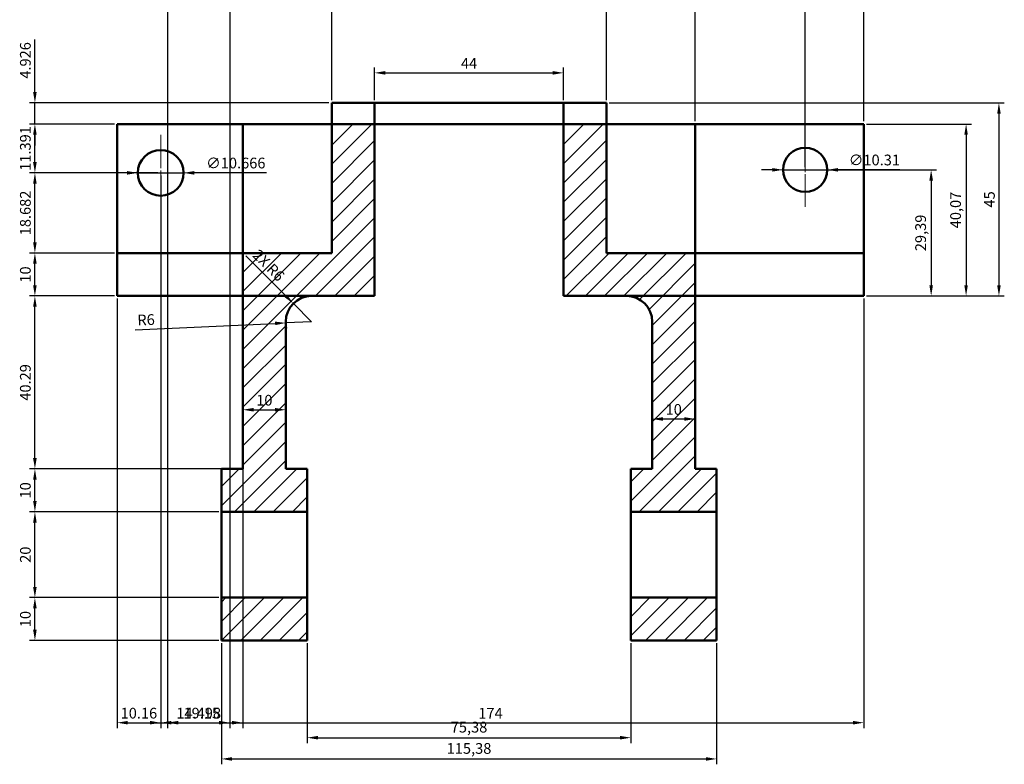
# Model space of a CAD drawing. Units: millimetres. Extents: x 2172 to 2566, y 897 to 1244.
# Tile 1 of 3: x 2172 to 2402, y 897 to 1071. Entities that reach past the tile are written whole.
import ezdxf

# ---------------------------------------------------------------- set-up
doc = ezdxf.new("R2010")
doc.units = ezdxf.units.MM
doc.linetypes.add('CENTER', pattern=[50.8, 31.75, -6.35, 6.35, -6.35])
for name, color, linetype, lineweight in [('M-CNTR', 4, 'CENTER', 18), ('M-DIMS', 2, 'Continuous', 25), ('M-HATC', 8, 'Continuous', 18), ('M-OUTL', 7, 'Continuous', 50)]:
    doc.layers.add(name, color=color, linetype=linetype, lineweight=lineweight)
doc.styles.get("Standard").update_dxf_attribs({"font": 'arial.ttf'})
doc.dimstyles.new('ISO-25', dxfattribs={"dimtxt": 2.5, "dimasz": 2.5, "dimexe": 1.25, "dimexo": 0.625, "dimtad": 1, "dimtxsty": 'Standard', "dimcen": 2.5, "dimadec": 0, "dimazin": 0, "dimtfac": 1, "dimtmove": 0, "dimatfit": 3, "dimfxl": 1, "dimarcsym": 0})

# ---------------------------------------------------------------- blocks, each defined once
blk = doc.blocks.new('*U1')
at = {"layer": 'M-CNTR', "color": 0, "transparency": 16777216}
for p, q in [((0, 1.07), (0, 8.83)), ((-8.83, 0), (-1.07, 0)), ((1.07, 0), (8.83, 0)), ((0, -8.83), (0, -1.07))]:
    blk.add_line(p, q, dxfattribs=at)
at = {"layer": 'M-CNTR', "color": 0, "linetype": 'Continuous', "transparency": 16777216}
for p, q in [((-0.53, 0), (0.53, 0)), ((0, -0.53), (0, 0.53))]:
    blk.add_line(p, q, dxfattribs=at)
blk = doc.blocks.new('*U2')
at = {"layer": 'M-CNTR', "color": 0, "transparency": 16777216}
for p, q in [((0, 1.03), (0, 8.66)), ((-8.66, 0), (-1.03, 0)), ((1.03, 0), (8.66, 0)), ((0, -8.66), (0, -1.03))]:
    blk.add_line(p, q, dxfattribs=at)
at = {"layer": 'M-CNTR', "color": 0, "linetype": 'Continuous', "transparency": 16777216}
for p, q in [((-0.52, 0), (0.52, 0)), ((0, -0.52), (0, 0.52))]:
    blk.add_line(p, q, dxfattribs=at)
blk = doc.blocks.new('*D10')
at = {"layer": 'Defpoints', "color": 0, "transparency": 16777216}
for p in [(2219.1, 925.96), (2334.48, 925.96), (2334.48, 898.37)]:
    blk.add_point(p, dxfattribs=at)
at = {"layer": 'M-DIMS', "color": 0, "lineweight": -2, "transparency": 16777216}
for p, q in [((2219.1, 925.34), (2219.1, 897.12)), ((2334.48, 925.34), (2334.48, 897.12)), ((2221.6, 898.37), (2331.98, 898.37))]:
    blk.add_line(p, q, dxfattribs=at)
at = {"layer": 'M-DIMS', "color": 0, "transparency": 16777216}
for points in [[(2221.6, 898.78), (2221.6, 897.95), (2219.1, 898.37)], [(2331.98, 898.78), (2331.98, 897.95), (2334.48, 898.37)]]:
    blk.add_solid(points, dxfattribs=at)
at = {"layer": 'M-DIMS', "color": 0, "transparency": 16777216, "insert": (2276.79, 900.49), "char_height": 2.5, "attachment_point": 5}
blk.add_mtext('115,38', dxfattribs=at)
blk = doc.blocks.new('*D11')
at = {"layer": 'Defpoints', "color": 0, "transparency": 16777216}
for p in [(2239.1, 925.96), (2314.48, 925.96), (2314.48, 903.32)]:
    blk.add_point(p, dxfattribs=at)
at = {"layer": 'M-DIMS', "color": 0, "lineweight": -2, "transparency": 16777216}
for p, q in [((2239.1, 925.34), (2239.1, 902.07)), ((2314.48, 925.34), (2314.48, 902.07)), ((2241.6, 903.32), (2311.98, 903.32))]:
    blk.add_line(p, q, dxfattribs=at)
at = {"layer": 'M-DIMS', "color": 0, "transparency": 16777216}
for points in [[(2241.6, 903.74), (2241.6, 902.9), (2239.1, 903.32)], [(2311.98, 903.74), (2311.98, 902.9), (2314.48, 903.32)]]:
    blk.add_solid(points, dxfattribs=at)
at = {"layer": 'M-DIMS', "color": 0, "transparency": 16777216, "insert": (2276.79, 905.45), "char_height": 2.5, "attachment_point": 5}
blk.add_mtext('75,38', dxfattribs=at)
blk = doc.blocks.new('*D12')
at = {"layer": 'Defpoints', "color": 0, "transparency": 16777216}
for p in [(2224.1, 986.11), (2234.1, 983.11), (2234.1, 979.74)]:
    blk.add_point(p, dxfattribs=at)
at = {"layer": 'M-DIMS', "color": 0, "lineweight": -2, "transparency": 16777216}
for p, q in [((2224.1, 985.48), (2224.1, 978.49)), ((2234.1, 982.48), (2234.1, 978.49)), ((2226.6, 979.74), (2231.6, 979.74))]:
    blk.add_line(p, q, dxfattribs=at)
at = {"layer": 'M-DIMS', "color": 0, "transparency": 16777216}
for points in [[(2226.6, 980.16), (2226.6, 979.32), (2224.1, 979.74)], [(2231.6, 980.16), (2231.6, 979.32), (2234.1, 979.74)]]:
    blk.add_solid(points, dxfattribs=at)
at = {"layer": 'M-DIMS', "color": 0, "transparency": 16777216, "insert": (2229.1, 981.64), "char_height": 2.5, "attachment_point": 5}
blk.add_mtext('10', dxfattribs=at)
blk = doc.blocks.new('*D13')
at = {"layer": 'Defpoints', "color": 0, "transparency": 16777216}
for p in [(2329.48, 986.11), (2319.48, 983.11), (2329.48, 977.59)]:
    blk.add_point(p, dxfattribs=at)
at = {"layer": 'M-DIMS', "color": 0, "lineweight": -2, "transparency": 16777216}
for p, q in [((2329.48, 985.48), (2329.48, 976.34)), ((2319.48, 982.48), (2319.48, 976.34)), ((2321.98, 977.59), (2326.98, 977.59))]:
    blk.add_line(p, q, dxfattribs=at)
at = {"layer": 'M-DIMS', "color": 0, "transparency": 16777216}
for points in [[(2321.98, 978.01), (2321.98, 977.17), (2319.48, 977.59)], [(2326.98, 978.01), (2326.98, 977.17), (2329.48, 977.59)]]:
    blk.add_solid(points, dxfattribs=at)
at = {"layer": 'M-DIMS', "color": 0, "transparency": 16777216, "insert": (2324.48, 979.49), "char_height": 2.5, "attachment_point": 5}
blk.add_mtext('10', dxfattribs=at)
blk = doc.blocks.new('*D14')
at = {"layer": 'Defpoints', "color": 0, "transparency": 16777216}
for p in [(2355.12, 1035.65), (2368.79, 1006.26), (2384.47, 1006.26)]:
    blk.add_point(p, dxfattribs=at)
at = {"layer": 'M-DIMS', "color": 0, "lineweight": -2, "transparency": 16777216}
for p, q in [((2355.75, 1035.65), (2385.72, 1035.65)), ((2384.47, 1033.15), (2384.47, 1008.76)), ((2369.41, 1006.26), (2385.72, 1006.26))]:
    blk.add_line(p, q, dxfattribs=at)
at = {"layer": 'M-DIMS', "color": 0, "transparency": 16777216}
for points in [[(2384.05, 1033.15), (2384.89, 1033.15), (2384.47, 1035.65)], [(2384.05, 1008.76), (2384.89, 1008.76), (2384.47, 1006.26)]]:
    blk.add_solid(points, dxfattribs=at)
at = {"layer": 'M-DIMS', "color": 0, "transparency": 16777216, "insert": (2382.34, 1020.95), "char_height": 2.5, "attachment_point": 5, "rotation": 90}
blk.add_mtext('29,39', dxfattribs=at)
blk = doc.blocks.new('*D15')
at = {"layer": 'Defpoints', "color": 0, "transparency": 16777216}
for p in [(2368.79, 1046.33), (2368.79, 1006.26), (2392.61, 1006.26)]:
    blk.add_point(p, dxfattribs=at)
at = {"layer": 'M-DIMS', "color": 0, "lineweight": -2, "transparency": 16777216}
for p, q in [((2369.41, 1046.33), (2393.86, 1046.33)), ((2392.61, 1043.83), (2392.61, 1008.76)), ((2369.41, 1006.26), (2393.86, 1006.26))]:
    blk.add_line(p, q, dxfattribs=at)
at = {"layer": 'M-DIMS', "color": 0, "transparency": 16777216}
for points in [[(2392.19, 1043.83), (2393.02, 1043.83), (2392.61, 1046.33)], [(2392.19, 1008.76), (2393.02, 1008.76), (2392.61, 1006.26)]]:
    blk.add_solid(points, dxfattribs=at)
at = {"layer": 'M-DIMS', "color": 0, "transparency": 16777216, "insert": (2390.48, 1026.29), "char_height": 2.5, "attachment_point": 5, "rotation": 90}
blk.add_mtext('40,07', dxfattribs=at)
blk = doc.blocks.new('*D16')
at = {"layer": 'Defpoints', "color": 0, "transparency": 16777216}
for p in [(2308.79, 1051.26), (2368.79, 1006.26), (2400.26, 1006.26)]:
    blk.add_point(p, dxfattribs=at)
at = {"layer": 'M-DIMS', "color": 0, "lineweight": -2, "transparency": 16777216}
for p, q in [((2309.41, 1051.26), (2401.51, 1051.26)), ((2400.26, 1048.76), (2400.26, 1008.76)), ((2369.41, 1006.26), (2401.51, 1006.26))]:
    blk.add_line(p, q, dxfattribs=at)
at = {"layer": 'M-DIMS', "color": 0, "transparency": 16777216}
for points in [[(2399.85, 1048.76), (2400.68, 1048.76), (2400.26, 1051.26)], [(2399.85, 1008.76), (2400.68, 1008.76), (2400.26, 1006.26)]]:
    blk.add_solid(points, dxfattribs=at)
at = {"layer": 'M-DIMS', "color": 0, "transparency": 16777216, "insert": (2398.37, 1028.76), "char_height": 2.5, "attachment_point": 5, "rotation": 90}
blk.add_mtext('45', dxfattribs=at)
blk = doc.blocks.new('*D17')
at = {"layer": 'Defpoints', "color": 0, "transparency": 16777216}
for p in [(2298.79, 1058.25), (2254.79, 1051.26), (2298.79, 1051.26)]:
    blk.add_point(p, dxfattribs=at)
at = {"layer": 'M-DIMS', "color": 0, "lineweight": -2, "transparency": 16777216}
for p, q in [((2254.79, 1051.88), (2254.79, 1059.5)), ((2257.29, 1058.25), (2296.29, 1058.25)), ((2298.79, 1051.88), (2298.79, 1059.5))]:
    blk.add_line(p, q, dxfattribs=at)
at = {"layer": 'M-DIMS', "color": 0, "transparency": 16777216}
for points in [[(2257.29, 1058.67), (2257.29, 1057.83), (2254.79, 1058.25)], [(2296.29, 1058.67), (2296.29, 1057.83), (2298.79, 1058.25)]]:
    blk.add_solid(points, dxfattribs=at)
at = {"layer": 'M-DIMS', "color": 0, "transparency": 16777216, "insert": (2276.79, 1060.13), "char_height": 2.5, "attachment_point": 5}
blk.add_mtext('44', dxfattribs=at)
blk = doc.blocks.new('*D18')
at = {"layer": 'Defpoints', "color": 0, "transparency": 16777216}
for p in [(2234.1, 999.98), (2240.1, 1000.26)]:
    blk.add_point(p, dxfattribs=at)
at = {"layer": 'M-DIMS', "color": 0, "lineweight": -2, "transparency": 16777216}
for p, q in [((2199, 998.36), (2231.61, 999.86)), ((2240.1, 1000.26), (2234.1, 999.98))]:
    blk.add_line(p, q, dxfattribs=at)
blk.add_arc((2240.1, 1000.26), 6, 180, 194.5824, dxfattribs=at)
at = {"layer": 'M-DIMS', "color": 0, "transparency": 16777216}
blk.add_solid([(2231.59, 1000.28), (2231.63, 999.45), (2234.1, 999.98)], dxfattribs=at)
at = {"layer": 'M-DIMS', "color": 0, "transparency": 16777216, "insert": (2201.55, 1000.38), "char_height": 2.5, "attachment_point": 5, "rotation": 2.6458}
blk.add_mtext('R6', dxfattribs=at)
blk = doc.blocks.new('*D40')
at = {"layer": 'Defpoints', "color": 0, "transparency": 16777216}
for p in [(2206.56, 1172.22), (2221.06, 1154.78), (2221.06, 906.81)]:
    blk.add_point(p, dxfattribs=at)
at = {"layer": 'M-DIMS', "color": 0, "lineweight": -2, "transparency": 16777216}
for p, q in [((2206.56, 1171.6), (2206.56, 905.56)), ((2221.06, 1154.15), (2221.06, 905.56)), ((2209.06, 906.81), (2218.56, 906.81))]:
    blk.add_line(p, q, dxfattribs=at)
at = {"layer": 'M-DIMS', "color": 0, "transparency": 16777216}
for points in [[(2209.06, 907.23), (2209.06, 906.4), (2206.56, 906.81)], [(2218.56, 907.23), (2218.56, 906.4), (2221.06, 906.81)]]:
    blk.add_solid(points, dxfattribs=at)
at = {"layer": 'M-DIMS', "color": 0, "transparency": 16777216, "insert": (2213.81, 908.71), "char_height": 2.5, "attachment_point": 5}
blk.add_mtext('14.498', dxfattribs=at)
blk = doc.blocks.new('*D41')
at = {"layer": 'Defpoints', "color": 0, "transparency": 16777216}
for p in [(2194.79, 1006.26), (2368.79, 1006.26), (2368.79, 906.81)]:
    blk.add_point(p, dxfattribs=at)
at = {"layer": 'M-DIMS', "color": 0, "lineweight": -2, "transparency": 16777216}
for p, q in [((2194.79, 1005.63), (2194.79, 905.56)), ((2368.79, 1005.63), (2368.79, 905.56)), ((2197.29, 906.81), (2366.29, 906.81))]:
    blk.add_line(p, q, dxfattribs=at)
at = {"layer": 'M-DIMS', "color": 0, "transparency": 16777216}
for points in [[(2197.29, 907.23), (2197.29, 906.4), (2194.79, 906.81)], [(2366.29, 907.23), (2366.29, 906.4), (2368.79, 906.81)]]:
    blk.add_solid(points, dxfattribs=at)
at = {"layer": 'M-DIMS', "color": 0, "transparency": 16777216, "insert": (2281.79, 908.69), "char_height": 2.5, "attachment_point": 5}
blk.add_mtext('174', dxfattribs=at)
blk = doc.blocks.new('*D42')
at = {"layer": 'Defpoints', "color": 0, "transparency": 16777216}
for p in [(2204.95, 1034.94), (2194.79, 1006.26), (2204.95, 906.81)]:
    blk.add_point(p, dxfattribs=at)
at = {"layer": 'M-DIMS', "color": 0, "lineweight": -2, "transparency": 16777216}
for p, q in [((2204.95, 1034.31), (2204.95, 905.56)), ((2194.79, 1005.63), (2194.79, 905.56)), ((2197.29, 906.81), (2202.45, 906.81))]:
    blk.add_line(p, q, dxfattribs=at)
at = {"layer": 'M-DIMS', "color": 0, "transparency": 16777216}
for points in [[(2197.29, 907.23), (2197.29, 906.4), (2194.79, 906.81)], [(2202.45, 907.23), (2202.45, 906.4), (2204.95, 906.81)]]:
    blk.add_solid(points, dxfattribs=at)
at = {"layer": 'M-DIMS', "color": 0, "transparency": 16777216, "insert": (2199.87, 908.71), "char_height": 2.5, "attachment_point": 5}
blk.add_mtext('10.16', dxfattribs=at)
blk = doc.blocks.new('*D43')
at = {"layer": 'Defpoints', "color": 0, "transparency": 16777216}
for p in [(2204.95, 1034.94), (2224.1, 1006.26), (2224.1, 906.81)]:
    blk.add_point(p, dxfattribs=at)
at = {"layer": 'M-DIMS', "color": 0, "lineweight": -2, "transparency": 16777216}
for p, q in [((2204.95, 1034.31), (2204.95, 905.56)), ((2224.1, 1005.63), (2224.1, 905.56)), ((2207.45, 906.81), (2221.6, 906.81))]:
    blk.add_line(p, q, dxfattribs=at)
at = {"layer": 'M-DIMS', "color": 0, "transparency": 16777216}
for points in [[(2207.45, 907.23), (2207.45, 906.4), (2204.95, 906.81)], [(2221.6, 907.23), (2221.6, 906.4), (2224.1, 906.81)]]:
    blk.add_solid(points, dxfattribs=at)
at = {"layer": 'M-DIMS', "color": 0, "transparency": 16777216, "insert": (2214.52, 908.71), "char_height": 2.5, "attachment_point": 5}
blk.add_mtext('19.15', dxfattribs=at)
blk = doc.blocks.new('*D44')
at = {"layer": 'Defpoints', "color": 0, "transparency": 16777216}
for p in [(2355.12, 1218.64), (2329.48, 1046.33), (2355.12, 1035.65)]:
    blk.add_point(p, dxfattribs=at)
at = {"layer": 'M-DIMS', "color": 0, "lineweight": -2, "transparency": 16777216}
for p, q in [((2329.48, 1046.96), (2329.48, 1219.89)), ((2331.98, 1218.64), (2352.62, 1218.64)), ((2355.12, 1036.27), (2355.12, 1219.89))]:
    blk.add_line(p, q, dxfattribs=at)
at = {"layer": 'M-DIMS', "color": 0, "transparency": 16777216}
for points in [[(2331.98, 1219.05), (2331.98, 1218.22), (2329.48, 1218.64)], [(2352.62, 1219.05), (2352.62, 1218.22), (2355.12, 1218.64)]]:
    blk.add_solid(points, dxfattribs=at)
at = {"layer": 'M-DIMS', "color": 0, "transparency": 16777216, "insert": (2342.3, 1220.54), "char_height": 2.5, "attachment_point": 5}
blk.add_mtext('25.643', dxfattribs=at)
blk = doc.blocks.new('*D45')
at = {"layer": 'Defpoints', "color": 0, "transparency": 16777216}
for p in [(2368.79, 1218.64), (2368.79, 1046.33), (2355.12, 1035.65)]:
    blk.add_point(p, dxfattribs=at)
at = {"layer": 'M-DIMS', "color": 0, "lineweight": -2, "transparency": 16777216}
for p, q in [((2355.12, 1036.27), (2355.12, 1219.89)), ((2357.62, 1218.64), (2366.29, 1218.64)), ((2368.79, 1046.96), (2368.79, 1219.89))]:
    blk.add_line(p, q, dxfattribs=at)
at = {"layer": 'M-DIMS', "color": 0, "transparency": 16777216}
for points in [[(2357.62, 1219.05), (2357.62, 1218.22), (2355.12, 1218.64)], [(2366.29, 1219.05), (2366.29, 1218.22), (2368.79, 1218.64)]]:
    blk.add_solid(points, dxfattribs=at)
at = {"layer": 'M-DIMS', "color": 0, "transparency": 16777216, "insert": (2361.95, 1220.54), "char_height": 2.5, "attachment_point": 5}
blk.add_mtext('13.668', dxfattribs=at)
blk = doc.blocks.new('*D46')
at = {"layer": 'Defpoints', "color": 0, "transparency": 16777216}
for p in [(2175.64, 935.96), (2219.1, 935.96), (2219.1, 925.96)]:
    blk.add_point(p, dxfattribs=at)
at = {"layer": 'M-DIMS', "color": 0, "lineweight": -2, "transparency": 16777216}
for p, q in [((2218.47, 935.96), (2174.39, 935.96)), ((2175.64, 928.46), (2175.64, 933.46)), ((2218.47, 925.96), (2174.39, 925.96))]:
    blk.add_line(p, q, dxfattribs=at)
at = {"layer": 'M-DIMS', "color": 0, "transparency": 16777216}
for points in [[(2175.22, 933.46), (2176.05, 933.46), (2175.64, 935.96)], [(2175.22, 928.46), (2176.05, 928.46), (2175.64, 925.96)]]:
    blk.add_solid(points, dxfattribs=at)
at = {"layer": 'M-DIMS', "color": 0, "transparency": 16777216, "insert": (2173.74, 930.96), "char_height": 2.5, "attachment_point": 5, "rotation": 90}
blk.add_mtext('10', dxfattribs=at)
blk = doc.blocks.new('*D47')
at = {"layer": 'Defpoints', "color": 0, "transparency": 16777216}
for p in [(2175.64, 955.96), (2219.1, 955.96), (2219.1, 935.96)]:
    blk.add_point(p, dxfattribs=at)
at = {"layer": 'M-DIMS', "color": 0, "lineweight": -2, "transparency": 16777216}
for p, q in [((2218.47, 955.96), (2174.39, 955.96)), ((2175.64, 938.46), (2175.64, 953.46)), ((2218.47, 935.96), (2174.39, 935.96))]:
    blk.add_line(p, q, dxfattribs=at)
at = {"layer": 'M-DIMS', "color": 0, "transparency": 16777216}
for points in [[(2175.22, 953.46), (2176.05, 953.46), (2175.64, 955.96)], [(2175.22, 938.46), (2176.05, 938.46), (2175.64, 935.96)]]:
    blk.add_solid(points, dxfattribs=at)
at = {"layer": 'M-DIMS', "color": 0, "transparency": 16777216, "insert": (2173.74, 945.96), "char_height": 2.5, "attachment_point": 5, "rotation": 90}
blk.add_mtext('20', dxfattribs=at)
blk = doc.blocks.new('*D48')
at = {"layer": 'Defpoints', "color": 0, "transparency": 16777216}
for p in [(2175.64, 965.96), (2219.1, 965.96), (2219.1, 955.96)]:
    blk.add_point(p, dxfattribs=at)
at = {"layer": 'M-DIMS', "color": 0, "lineweight": -2, "transparency": 16777216}
for p, q in [((2218.47, 965.96), (2174.39, 965.96)), ((2175.64, 958.46), (2175.64, 963.46)), ((2218.47, 955.96), (2174.39, 955.96))]:
    blk.add_line(p, q, dxfattribs=at)
at = {"layer": 'M-DIMS', "color": 0, "transparency": 16777216}
for points in [[(2175.22, 963.46), (2176.05, 963.46), (2175.64, 965.96)], [(2175.22, 958.46), (2176.05, 958.46), (2175.64, 955.96)]]:
    blk.add_solid(points, dxfattribs=at)
at = {"layer": 'M-DIMS', "color": 0, "transparency": 16777216, "insert": (2173.74, 960.96), "char_height": 2.5, "attachment_point": 5, "rotation": 90}
blk.add_mtext('10', dxfattribs=at)
blk = doc.blocks.new('*D49')
at = {"layer": 'Defpoints', "color": 0, "transparency": 16777216}
for p in [(2175.64, 1006.26), (2194.79, 1006.26), (2224.1, 965.96)]:
    blk.add_point(p, dxfattribs=at)
at = {"layer": 'M-DIMS', "color": 0, "lineweight": -2, "transparency": 16777216}
for p, q in [((2194.16, 1006.26), (2174.39, 1006.26)), ((2175.64, 968.46), (2175.64, 1003.76)), ((2223.47, 965.96), (2174.39, 965.96))]:
    blk.add_line(p, q, dxfattribs=at)
at = {"layer": 'M-DIMS', "color": 0, "transparency": 16777216}
for points in [[(2175.22, 1003.76), (2176.05, 1003.76), (2175.64, 1006.26)], [(2175.22, 968.46), (2176.05, 968.46), (2175.64, 965.96)]]:
    blk.add_solid(points, dxfattribs=at)
at = {"layer": 'M-DIMS', "color": 0, "transparency": 16777216, "insert": (2173.74, 986.11), "char_height": 2.5, "attachment_point": 5, "rotation": 90}
blk.add_mtext('40.29', dxfattribs=at)
blk = doc.blocks.new('*D50')
at = {"layer": 'Defpoints', "color": 0, "transparency": 16777216}
for p in [(2175.64, 1016.26), (2194.79, 1016.26), (2194.79, 1006.26)]:
    blk.add_point(p, dxfattribs=at)
at = {"layer": 'M-DIMS', "color": 0, "lineweight": -2, "transparency": 16777216}
for p, q in [((2194.16, 1016.26), (2174.39, 1016.26)), ((2175.64, 1008.76), (2175.64, 1013.76)), ((2194.16, 1006.26), (2174.39, 1006.26))]:
    blk.add_line(p, q, dxfattribs=at)
at = {"layer": 'M-DIMS', "color": 0, "transparency": 16777216}
for points in [[(2175.22, 1013.76), (2176.05, 1013.76), (2175.64, 1016.26)], [(2175.22, 1008.76), (2176.05, 1008.76), (2175.64, 1006.26)]]:
    blk.add_solid(points, dxfattribs=at)
at = {"layer": 'M-DIMS', "color": 0, "transparency": 16777216, "insert": (2173.74, 1011.26), "char_height": 2.5, "attachment_point": 5, "rotation": 90}
blk.add_mtext('10', dxfattribs=at)
blk = doc.blocks.new('*D51')
at = {"layer": 'Defpoints', "color": 0, "transparency": 16777216}
for p in [(2175.64, 1034.94), (2204.95, 1034.94), (2194.79, 1016.26)]:
    blk.add_point(p, dxfattribs=at)
at = {"layer": 'M-DIMS', "color": 0, "lineweight": -2, "transparency": 16777216}
for p, q in [((2204.32, 1034.94), (2174.39, 1034.94)), ((2175.64, 1018.76), (2175.64, 1032.44)), ((2194.16, 1016.26), (2174.39, 1016.26))]:
    blk.add_line(p, q, dxfattribs=at)
at = {"layer": 'M-DIMS', "color": 0, "transparency": 16777216}
for points in [[(2175.22, 1032.44), (2176.05, 1032.44), (2175.64, 1034.94)], [(2175.22, 1018.76), (2176.05, 1018.76), (2175.64, 1016.26)]]:
    blk.add_solid(points, dxfattribs=at)
at = {"layer": 'M-DIMS', "color": 0, "transparency": 16777216, "insert": (2173.74, 1025.6), "char_height": 2.5, "attachment_point": 5, "rotation": 90}
blk.add_mtext('18.682', dxfattribs=at)
blk = doc.blocks.new('*D52')
at = {"layer": 'Defpoints', "color": 0, "transparency": 16777216}
for p in [(2175.64, 1046.33), (2194.79, 1046.33), (2204.95, 1034.94)]:
    blk.add_point(p, dxfattribs=at)
at = {"layer": 'M-DIMS', "color": 0, "lineweight": -2, "transparency": 16777216}
for p, q in [((2194.16, 1046.33), (2174.39, 1046.33)), ((2175.64, 1037.44), (2175.64, 1043.83)), ((2204.32, 1034.94), (2174.39, 1034.94))]:
    blk.add_line(p, q, dxfattribs=at)
at = {"layer": 'M-DIMS', "color": 0, "transparency": 16777216}
for points in [[(2175.22, 1043.83), (2176.05, 1043.83), (2175.64, 1046.33)], [(2175.22, 1037.44), (2176.05, 1037.44), (2175.64, 1034.94)]]:
    blk.add_solid(points, dxfattribs=at)
at = {"layer": 'M-DIMS', "color": 0, "transparency": 16777216, "insert": (2173.74, 1040.63), "char_height": 2.5, "attachment_point": 5, "rotation": 90}
blk.add_mtext('11.391', dxfattribs=at)
blk = doc.blocks.new('*D53')
at = {"layer": 'Defpoints', "color": 0, "transparency": 16777216}
for p in [(2175.64, 1051.26), (2244.79, 1051.26), (2194.79, 1046.33)]:
    blk.add_point(p, dxfattribs=at)
at = {"layer": 'M-DIMS', "color": 0, "lineweight": -2, "transparency": 16777216}
for p, q in [((2175.64, 1053.76), (2175.64, 1066.04)), ((2244.16, 1051.26), (2174.39, 1051.26)), ((2175.64, 1046.33), (2175.64, 1051.26)), ((2194.16, 1046.33), (2174.39, 1046.33)), ((2175.64, 1043.83), (2175.64, 1041.33))]:
    blk.add_line(p, q, dxfattribs=at)
at = {"layer": 'M-DIMS', "color": 0, "transparency": 16777216}
for points in [[(2175.22, 1053.76), (2176.05, 1053.76), (2175.64, 1051.26)], [(2175.22, 1043.83), (2176.05, 1043.83), (2175.64, 1046.33)]]:
    blk.add_solid(points, dxfattribs=at)
at = {"layer": 'M-DIMS', "color": 0, "transparency": 16777216, "insert": (2173.74, 1061.15), "char_height": 2.5, "attachment_point": 5, "rotation": 90}
blk.add_mtext('4.926', dxfattribs=at)
blk = doc.blocks.new('*D54')
at = {"layer": 'Defpoints', "color": 0, "transparency": 16777216}
for p in [(2308.79, 1218.64), (2244.79, 1051.26), (2308.79, 1051.26)]:
    blk.add_point(p, dxfattribs=at)
at = {"layer": 'M-DIMS', "color": 0, "lineweight": -2, "transparency": 16777216}
for p, q in [((2244.79, 1051.88), (2244.79, 1219.89)), ((2247.29, 1218.64), (2306.29, 1218.64)), ((2308.79, 1051.88), (2308.79, 1219.89))]:
    blk.add_line(p, q, dxfattribs=at)
at = {"layer": 'M-DIMS', "color": 0, "transparency": 16777216}
for points in [[(2247.29, 1219.05), (2247.29, 1218.22), (2244.79, 1218.64)], [(2306.29, 1219.05), (2306.29, 1218.22), (2308.79, 1218.64)]]:
    blk.add_solid(points, dxfattribs=at)
at = {"layer": 'M-DIMS', "color": 0, "transparency": 16777216, "insert": (2276.79, 1220.54), "char_height": 2.5, "attachment_point": 5}
blk.add_mtext('64', dxfattribs=at)
blk = doc.blocks.new('*D68')
at = {"layer": 'Defpoints', "color": 0, "transparency": 16777216}
for p in [(2235.86, 1004.5), (2240.1, 1000.26)]:
    blk.add_point(p, dxfattribs=at)
at = {"layer": 'M-DIMS', "color": 0, "lineweight": -2, "transparency": 16777216}
for p, q in [((2224.76, 1015.6), (2234.09, 1006.27)), ((2240.1, 1000.26), (2235.86, 1004.5))]:
    blk.add_line(p, q, dxfattribs=at)
at = {"layer": 'M-DIMS', "color": 0, "transparency": 16777216}
blk.add_solid([(2234.38, 1006.56), (2233.79, 1005.97), (2235.86, 1004.5)], dxfattribs=at)
at = {"layer": 'M-DIMS', "color": 0, "transparency": 16777216, "insert": (2229.88, 1013.16), "char_height": 2.5, "attachment_point": 5, "rotation": 314.9983}
blk.add_mtext('2X R6', dxfattribs=at)
blk = doc.blocks.new('*D69')
at = {"layer": 'Defpoints', "color": 0, "transparency": 16777216}
for p in [(2199.61, 1034.94), (2210.28, 1034.94)]:
    blk.add_point(p, dxfattribs=at)
at = {"layer": 'M-DIMS', "color": 0, "lineweight": -2, "transparency": 16777216}
for p, q in [((2197.11, 1034.94), (2194.61, 1034.94)), ((2199.61, 1034.94), (2210.28, 1034.94)), ((2229.63, 1034.94), (2212.78, 1034.94))]:
    blk.add_line(p, q, dxfattribs=at)
at = {"layer": 'M-DIMS', "color": 0, "transparency": 16777216}
for points in [[(2197.11, 1035.36), (2197.11, 1034.52), (2199.61, 1034.94)], [(2212.78, 1035.36), (2212.78, 1034.52), (2210.28, 1034.94)]]:
    blk.add_solid(points, dxfattribs=at)
at = {"layer": 'M-DIMS', "color": 0, "transparency": 16777216, "insert": (2222.45, 1036.91), "char_height": 2.5, "attachment_point": 5, "rotation": 0.0014}
blk.add_mtext('∅10.666', dxfattribs=at)
blk = doc.blocks.new('*D70')
at = {"layer": 'Defpoints', "color": 0, "transparency": 16777216}
for p in [(2349.96, 1035.65), (2360.28, 1035.65)]:
    blk.add_point(p, dxfattribs=at)
at = {"layer": 'M-DIMS', "color": 0, "lineweight": -2, "transparency": 16777216}
for p, q in [((2347.46, 1035.65), (2344.96, 1035.65)), ((2349.96, 1035.65), (2360.28, 1035.65)), ((2377.2, 1035.65), (2362.78, 1035.65))]:
    blk.add_line(p, q, dxfattribs=at)
at = {"layer": 'M-DIMS', "color": 0, "transparency": 16777216}
for points in [[(2347.46, 1036.07), (2347.46, 1035.23), (2349.96, 1035.65)], [(2362.78, 1036.07), (2362.78, 1035.23), (2360.28, 1035.65)]]:
    blk.add_solid(points, dxfattribs=at)
at = {"layer": 'M-DIMS', "color": 0, "transparency": 16777216, "insert": (2371.24, 1037.62), "char_height": 2.5, "attachment_point": 5, "rotation": 0.0004}
blk.add_mtext('∅10.31', dxfattribs=at)

msp = doc.modelspace()

# ---------------------------------------------------------------- hatches: boundary and pattern name
at = {"layer": 'M-HATC'}
h = msp.add_hatch(dxfattribs=at)
h.set_pattern_fill('ANSI31', color=256)
h.paths.add_polyline_path([(2239.0983, 965.9626), (2234.0983, 965.9626), (2234.0983, 1000.2565, -0.41421356), (2240.0983, 1006.2565), (2224.0983, 1006.2565), (2224.0983, 965.9626), (2219.0983, 965.9626), (2219.0983, 955.9626), (2239.0983, 955.9626)])
h.paths.add_polyline_path([(2254.7875, 1046.3302), (2244.7875, 1046.3302), (2244.7875, 1016.2565), (2224.0983, 1016.2565), (2224.0983, 1006.2565), (2240.0983, 1006.2565), (2254.7875, 1006.2565)])
h.paths.add_polyline_path([(2308.7875, 1046.3302), (2298.7875, 1046.3302), (2298.7875, 1006.2565), (2313.4768, 1006.2565), (2329.4768, 1006.2565), (2329.4768, 1016.2565), (2308.7875, 1016.2565)])
h.paths.add_polyline_path([(2329.4768, 1006.2565), (2313.4768, 1006.2565, -0.41421356), (2319.4768, 1000.2565), (2319.4768, 965.9626), (2314.4768, 965.9626), (2314.4768, 955.9626), (2334.4768, 955.9626), (2334.4768, 965.9626), (2329.4768, 965.9626)])
h.paths.add_polyline_path([(2334.4768, 935.9626), (2314.4768, 935.9626), (2314.4768, 925.9626), (2334.4768, 925.9626)])
h.paths.add_polyline_path([(2239.0983, 935.9626), (2219.0983, 935.9626), (2219.0983, 925.9626), (2239.0983, 925.9626)])

# ---------------------------------------------------------------- linework, layer by layer
at = {"layer": 'M-OUTL'}
for p, q in [((2276.7875, 1051.2565), (2244.7875, 1051.2565)), ((2244.7875, 1051.2565), (2244.7875, 1016.2565)), ((2254.7875, 1006.2565), (2254.7875, 1051.2565)), ((2276.7875, 1051.2565), (2308.7875, 1051.2565)), ((2298.7875, 1006.2565), (2298.7875, 1051.2565)), ((2308.7875, 1051.2565), (2308.7875, 1016.2565)), ((2194.7875, 1016.2565), (2194.7875, 1046.3302)), ((2368.7875, 1046.3302), (2194.7875, 1046.3302)), ((2224.0983, 1006.2565), (2224.0983, 1046.3302)), ((2329.4768, 1006.2565), (2329.4768, 1046.3302)), ((2368.7875, 1016.2565), (2368.7875, 1046.3302)), ((2244.7875, 1016.2565), (2194.7875, 1016.2565)), ((2194.7875, 1016.2565), (2194.7875, 1006.2565)), ((2308.7875, 1016.2565), (2368.7875, 1016.2565)), ((2368.7875, 1016.2565), (2368.7875, 1006.2565)), ((2194.7875, 1006.2565), (2224.0983, 1006.2565)), ((2224.0983, 1006.2565), (2224.0983, 965.9626)), ((2224.0983, 1006.2565), (2240.0983, 1006.2565)), ((2240.0983, 1006.2565), (2254.7875, 1006.2565)), ((2313.4768, 1006.2565), (2298.7875, 1006.2565)), ((2313.4768, 1006.2565), (2329.4768, 1006.2565)), ((2329.4768, 1006.2565), (2329.4768, 965.9626)), ((2329.4768, 1006.2565), (2339.5539, 1006.2565)), ((2339.5539, 1006.2565), (2368.7875, 1006.2565)), ((2234.0983, 965.9626), (2234.0983, 1000.2565)), ((2319.4768, 965.9626), (2319.4768, 1000.2565)), ((2224.0983, 965.9626), (2219.0983, 965.9626)), ((2219.0983, 965.9626), (2219.0983, 925.9626)), ((2239.0983, 965.9626), (2234.0983, 965.9626)), ((2239.0983, 925.9626), (2239.0983, 965.9626)), ((2314.4768, 925.9626), (2314.4768, 965.9626)), ((2314.4768, 965.9626), (2319.4768, 965.9626)), ((2329.4768, 965.9626), (2334.4768, 965.9626)), ((2334.4768, 965.9626), (2334.4768, 925.9626)), ((2219.0983, 955.9626), (2239.0983, 955.9626)), ((2314.4768, 955.9626), (2334.4768, 955.9626)), ((2239.0983, 935.9626), (2219.0983, 935.9626)), ((2239.0983, 925.9626), (2239.0983, 935.9626)), ((2334.4768, 935.9626), (2314.4768, 935.9626)), ((2219.0983, 925.9626), (2239.0983, 925.9626)), ((2334.4768, 925.9626), (2314.4768, 925.9626))]:
    msp.add_line(p, q, dxfattribs=at)
for centre, radius in [((2204.9477, 1034.9389), 5.3332), ((2355.12, 1035.65), 5.1554)]:
    msp.add_circle(centre, radius, dxfattribs=at)
for centre, start, end in [((2240.0983, 1000.2565), 90, 180), ((2313.4768, 1000.2565), 0, 90)]:
    msp.add_arc(centre, 6, start, end, dxfattribs=at)

# ---------------------------------------------------------------- block references
at = {"layer": 'M-CNTR'}
for name, p in [('*U2', (2355.12, 1035.65)), ('*U1', (2204.9477, 1034.9389))]:
    msp.add_blockref(name, p, dxfattribs=at)

# ---------------------------------------------------------------- dimensions: what is measured, and where the dimension line sits
at = {"layer": 'M-DIMS'}
for base, p1, p2, override, picture, middle in [((2308.7875, 1218.6372), (2244.7875, 1051.2565), (2308.7875, 1051.2565), {"dimdec": 0, "dimlfac": 1, "dimrnd": 0, "dimzin": 0, "dimdsep": 46, "dimlunit": 2}, '*D54', (2276.7875, 1220.5386)), ((2355.12, 1218.6372), (2329.4768, 1046.3302), (2355.12, 1035.65), {"dimdec": 3, "dimlfac": 1, "dimrnd": 0, "dimzin": 0, "dimdsep": 46, "dimlunit": 2}, '*D44', (2342.2984, 1220.5395)), ((2368.78755, 1218.63717), (2355.12001, 1035.64997), (2368.78755, 1046.33023), {"dimdec": 3, "dimlfac": 1, "dimrnd": 0, "dimzin": 0, "dimdsep": 46, "dimlunit": 2}, '*D45', (2361.95378, 1220.53946)), ((2221.059, 906.8126), (2206.5611, 1172.2234), (2221.059, 1154.7754), {"dimdec": 3, "dimlfac": 1, "dimrnd": 0, "dimzin": 0, "dimdsep": 46, "dimlunit": 2}, '*D40', (2213.81, 908.714)), ((2298.7875, 1058.2516), (2254.7875, 1051.2565), (2298.7875, 1051.2565), {"dimclrd": 0, "dimclre": 0, "dimclrt": 0}, '*D17', (2276.7875, 1060.1266)), ((2204.9477, 906.8126), (2194.7875, 1006.2565), (2204.9477, 1034.9389), {"dimdec": 2, "dimlfac": 1, "dimrnd": 0, "dimzin": 0, "dimdsep": 46, "dimlunit": 2}, '*D42', (2199.8676, 908.714)), ((2224.0983, 906.8126), (2204.9477, 1034.9389), (2224.0983, 1006.2565), {"dimdec": 2, "dimlfac": 1, "dimrnd": 0, "dimzin": 0, "dimdsep": 46, "dimlunit": 2}, '*D43', (2214.523, 908.714)), ((2368.7875, 906.8126), (2194.7875, 1006.2565), (2368.7875, 1006.2565), {"dimdec": 0, "dimlfac": 1, "dimrnd": 0, "dimzin": 0, "dimdsep": 46, "dimlunit": 2}, '*D41', (2281.7875, 908.6927)), ((2234.0983, 979.7415), (2224.0983, 986.1095), (2234.0983, 983.1095), {"dimclrd": 0, "dimclre": 0, "dimclrt": 0}, '*D12', (2229.0983, 981.6429)), ((2329.4768, 977.5897), (2319.4768, 983.1095), (2329.4768, 986.1095), {"dimclrd": 0, "dimclre": 0, "dimclrt": 0}, '*D13', (2324.4768, 979.4911)), ((2334.4768, 898.3654), (2219.0983, 925.9626), (2334.4768, 925.9626), {"dimclrd": 0, "dimclre": 0, "dimclrt": 0}, '*D10', (2276.7875, 900.4928)), ((2314.4768, 903.3209), (2239.0983, 925.9626), (2314.4768, 925.9626), {"dimclrd": 0, "dimclre": 0, "dimclrt": 0}, '*D11', (2276.7875, 905.4483))]:
    dim = msp.add_linear_dim(base=base, p1=p1, p2=p2, dimstyle='ISO-25', override=override, dxfattribs=at)
    dim.commit()
    dim.dimension.update_dxf_attribs({"geometry": picture, "text_midpoint": middle})
for base, p1, p2, override, picture, middle in [((2175.6375, 1051.2565), (2194.7875, 1046.3302), (2244.7875, 1051.2565), {"dimdec": 3, "dimlfac": 1, "dimrnd": 0, "dimzin": 0, "dimdsep": 46, "dimlunit": 2}, '*D53', (2173.7361, 1061.1491)), ((2400.2635, 1006.2565), (2308.7875, 1051.2565), (2368.7875, 1006.2565), {"dimclrd": 0, "dimclre": 0, "dimclrt": 0}, '*D16', (2398.3672, 1028.7565)), ((2175.6375, 1046.3302), (2204.9477, 1034.9389), (2194.7875, 1046.3302), {"dimdec": 3, "dimlfac": 1, "dimrnd": 0, "dimzin": 0, "dimdsep": 46, "dimlunit": 2}, '*D52', (2173.7353, 1040.6346)), ((2392.606, 1006.2565), (2368.7875, 1046.3302), (2368.7875, 1006.2565), {"dimclrd": 0, "dimclre": 0, "dimclrt": 0}, '*D15', (2390.4786, 1026.2934)), ((2175.6375, 1034.9389), (2194.7875, 1016.2565), (2204.9477, 1034.9389), {"dimdec": 3, "dimlfac": 1, "dimrnd": 0, "dimzin": 0, "dimdsep": 46, "dimlunit": 2}, '*D51', (2173.7361, 1025.5977)), ((2384.4698, 1006.2565), (2355.12, 1035.65), (2368.7875, 1006.2565), {"dimclrd": 0, "dimclre": 0, "dimclrt": 0}, '*D14', (2382.3424, 1020.9532)), ((2175.6375, 1016.2565), (2194.7875, 1006.2565), (2194.7875, 1016.2565), {"dimdec": 0, "dimlfac": 1, "dimrnd": 0, "dimzin": 0, "dimdsep": 46, "dimlunit": 2}, '*D50', (2173.7361, 1011.2565)), ((2175.6375, 1006.2565), (2224.0983, 965.9626), (2194.7875, 1006.2565), {"dimdec": 2, "dimlfac": 1, "dimrnd": 0, "dimzin": 0, "dimdsep": 46, "dimlunit": 2}, '*D49', (2173.7361, 986.1095)), ((2175.6375, 965.9626), (2219.0983, 955.9626), (2219.0983, 965.9626), {"dimdec": 0, "dimlfac": 1, "dimrnd": 0, "dimzin": 0, "dimdsep": 46, "dimlunit": 2}, '*D48', (2173.7361, 960.9626)), ((2175.6375, 955.9626), (2219.0983, 935.9626), (2219.0983, 955.9626), {"dimdec": 0, "dimlfac": 1, "dimrnd": 0, "dimzin": 0, "dimdsep": 46, "dimlunit": 2}, '*D47', (2173.7361, 945.9626)), ((2175.6375, 935.9626), (2219.0983, 925.9626), (2219.0983, 935.9626), {"dimdec": 0, "dimlfac": 1, "dimrnd": 0, "dimzin": 0, "dimdsep": 46, "dimlunit": 2}, '*D46', (2173.7361, 930.9626))]:
    dim = msp.add_linear_dim(base=base, p1=p1, p2=p2, angle=90, dimstyle='ISO-25', override=override, dxfattribs=at)
    dim.commit()
    dim.dimension.update_dxf_attribs({"geometry": picture, "text_midpoint": middle})
dim = msp.add_diameter_dim_2p(p1=(2199.61445, 1034.93874), p2=(2210.28087, 1034.939), dimstyle='ISO-25', override={"dimdec": 3, "dimlfac": 1, "dimrnd": 0, "dimzin": 0, "dimdsep": 46, "dimlunit": 2}, dxfattribs=at)
dim.commit()
dim.dimension.update_dxf_attribs({"geometry": '*D69', "text_midpoint": (2222.4543, 1034.9393)})
dim = msp.add_diameter_dim_2p(p1=(2349.9646, 1035.6499), p2=(2360.2754, 1035.65), dimstyle='ISO-25', override={"dimdec": 2, "dimlfac": 1, "dimrnd": 0, "dimzin": 0, "dimdsep": 46, "dimlunit": 2}, dxfattribs=at)
dim.commit()
dim.dimension.update_dxf_attribs({"geometry": '*D70', "text_midpoint": (2371.2372, 1035.6501), "dimtype": 163})
dim = msp.add_radius_dim(center=(2240.0983, 1000.2565), mpoint=(2235.8557, 1004.4993), text='2X <>', dimstyle='ISO-25', override={"dimdec": 0, "dimlfac": 1, "dimrnd": 0, "dimzin": 0, "dimdsep": 46, "dimlunit": 2}, dxfattribs=at)
dim.commit()
dim.dimension.update_dxf_attribs({"geometry": '*D68', "text_midpoint": (2229.884, 1013.1604)})
dim = msp.add_radius_dim(center=(2240.0983, 1000.2565), mpoint=(2234.1046, 999.9795), dimstyle='ISO-25', override={"dimclrd": 0, "dimclre": 0, "dimclrt": 0}, dxfattribs=at)
dim.commit()
dim.dimension.update_dxf_attribs({"geometry": '*D18', "text_midpoint": (2201.637, 998.4792), "dimtype": 164})

doc.saveas('drawing.dxf')
